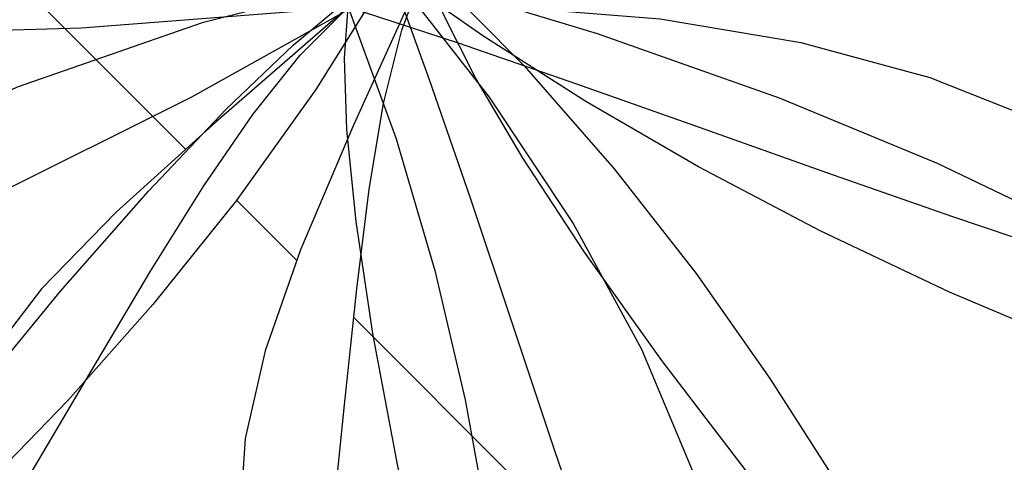
# Model space of a CAD drawing. Units: inches. Extents: x 3590 to 5167, y 65 to 1917.
# Tile 74 of 100: x 5045.84 to 5058.39, y 1773.22 to 1778.86. Entities that reach past the tile are written whole.
import ezdxf

# ---------------------------------------------------------------- set-up
doc = ezdxf.new("R2010")
doc.units = ezdxf.units.IN
for name, color, linetype, lineweight in [('A-ANNO-DIMS', 2, 'Continuous', 18), ('A-FLOR-PATT', 8, 'Continuous', 13), ('L-PLNT', 94, 'Continuous', 18)]:
    doc.layers.add(name, color=color, linetype=linetype, lineweight=lineweight)
doc.layers.add('DIENHOA', color=3, linetype='Continuous')
doc.styles.get("Standard").update_dxf_attribs({"font": 'arial.ttf'})
doc.dimstyles.new('ISO-25', dxfattribs={"dimtxt": 9, "dimasz": 2.5, "dimexe": 1.25, "dimexo": 0.625, "dimtad": 1, "dimdec": 1, "dimlunit": 3, "dimtxsty": 'Standard', "dimcen": 2.5, "dimadec": 0, "dimazin": 0, "dimtfac": 1, "dimtdec": 1, "dimtmove": 0, "dimatfit": 3, "dimfxl": 1, "dimarcsym": 0})

# ---------------------------------------------------------------- blocks, each defined once
blk = doc.blocks.new('Cay03_mb')
at = {"layer": 'DIENHOA'}
for p, q in [((5.39, -7.78), (-33.18, -69.47)), ((5.39, -7.78), (56.83, -73.35)), ((25.88, -64.38), (5.39, -7.78)), ((5.39, -7.78), (112.81, -40.3)), ((53.47, -41.58), (5.39, -7.78)), ((-45.06, -46.34), (-16.51, -22.43)), ((112.81, -40.3), (207.46, -73.81)), ((106.98, -75.69), (53.47, -41.58)), ((-79.78, -79.55), (-45.06, -46.34)), ((47.05, -125.9), (25.88, -64.38)), ((-33.18, -69.47), (-74.57, -127.29)), ((56.83, -73.35), (100.42, -139.07)), ((165.52, -109.6), (106.98, -75.69)), ((207.46, -73.81), (289.55, -107.64)), ((-120.2, -122.13), (-79.78, -79.55)), ((228.67, -142.77), (165.52, -109.6)), ((289.55, -107.64), (359.29, -141.1)), ((-165.86, -174.12), (-120.2, -122.13)), ((-74.57, -127.29), (-117.85, -181.14)), ((68.74, -190.55), (47.05, -125.9)), ((100.42, -139.07), (135.85, -204.28)), ((296, -174.69), (228.67, -142.77)), ((-216.28, -235.58), (-165.86, -174.12)), ((367.1, -204.83), (296, -174.69)), ((-117.85, -181.14), (-162.07, -230.91)), ((90.79, -256.57), (68.74, -190.55)), ((135.85, -204.28), (162.8, -268.28)), ((-162.07, -230.91), (-206.29, -276.49)), ((113.06, -322.16), (90.79, -256.57))]:
    blk.add_line(p, q, dxfattribs=at)
for points in [[(-471.89, -320.34), (-310.46, -179.32), (-97.66, -73.3), (23.69, -5.44)], [(23.69, -5.44), (-92.3, -34.76), (-188.42, -68.2), (-266.88, -105.14), (-329.9, -144.95), (-379.7, -187), (-418.48, -230.67), (-448.47, -275.32), (-471.89, -320.34)], [(23.69, -5.44), (-13.63, -87.94), (-41.14, -152.63), (-59.64, -205.04), (-69.94, -250.66), (-72.84, -295), (-69.17, -343.58), (-59.73, -401.89), (-45.32, -475.45)], [(-45.32, -475.45), (-34.09, -383.24), (-25.4, -302.82), (-18.34, -233.08), (-12.02, -172.9), (-5.55, -121.16), (1.96, -76.75), (11.41, -38.55), (23.69, -5.44)], [(316.49, -418.14), (251.44, -342.76), (194.84, -273.28), (146.52, -210.16), (106.33, -153.83), (74.11, -104.75), (49.71, -63.36), (32.95, -30.11), (23.69, -5.44)], [(23.69, -5.44), (74.94, -57.08), (121.78, -110.58), (164.32, -165.02), (202.67, -219.43), (236.95, -272.89), (267.27, -324.46), (293.75, -373.19), (316.49, -418.14)], [(-598.36, -104.66), (-392.67, -44.38), (-155.01, -37.42), (-16.39, -26.73)], [(-276.22, -424.43), (-227.35, -345.43), (-185.71, -276.08), (-150.05, -215.74), (-119.06, -163.76), (-91.49, -119.51), (-66.04, -82.35), (-41.43, -51.64), (-16.39, -26.73)], [(-16.39, -26.73), (-84.88, -85.96), (-136.99, -133.15), (-175.77, -172.96), (-204.26, -210.05), (-225.5, -249.08), (-242.55, -294.71), (-258.44, -351.61), (-276.22, -424.43)], [(76.25, -524.2), (48.83, -428.48), (26.6, -341.67), (9.22, -264.1), (-3.63, -196.11), (-12.28, -138.04), (-17.07, -90.23), (-18.33, -53.01), (-16.39, -26.73)], [(-16.39, -26.73), (66.95, -26.58), (145.58, -32.71), (218.77, -44.94), (285.79, -63.12), (345.92, -87.06), (398.42, -116.6), (442.57, -151.57), (477.63, -191.79)], [(477.63, -191.79), (421.82, -176.03), (361.32, -156.94), (297.62, -135.49), (232.22, -112.64), (166.63, -89.37), (102.33, -66.65), (40.82, -45.45), (-16.39, -26.73)], [(-16.39, -26.73), (8.47, -95.11), (28.54, -163.33), (44.32, -230.59), (56.3, -296.08), (64.99, -358.99), (70.88, -418.52), (74.46, -473.86), (76.25, -524.2)]]:
    blk.add_lwpolyline(points, dxfattribs=at)
blk = doc.blocks.new('*D322')
at = {"layer": 'A-ANNO-DIMS', "color": 0, "lineweight": -2, "transparency": 16777216}
for p, q in [((5035.744, 1766.184), (5035.744, 1761.199)), ((5064.812, 1766.184), (5064.812, 1761.199)), ((5038.244, 1762.449), (5062.312, 1762.449)), ((5064.812, 1762.449), (5166.991, 1762.449))]:
    blk.add_line(p, q, dxfattribs=at)
at = {"layer": 'A-ANNO-DIMS', "color": 0, "transparency": 16777216}
for points in [[(5038.244, 1762.866), (5038.244, 1762.032), (5035.744, 1762.449)], [(5062.312, 1762.866), (5062.312, 1762.032), (5064.812, 1762.449)]]:
    blk.add_solid(points, dxfattribs=at)
at = {"layer": 'Defpoints', "color": 0, "transparency": 16777216}
for p in [(5035.744, 1766.809), (5064.812, 1766.809), (5064.812, 1762.449)]:
    blk.add_point(p, dxfattribs=at)
at = {"layer": 'A-ANNO-DIMS', "color": 0, "transparency": 16777216, "insert": (5117.152, 1767.669), "char_height": 9, "attachment_point": 5}
blk.add_mtext('PLANT 2\'-5" TYP.', dxfattribs=at)
blk = doc.blocks.new('*D323')
at = {"layer": 'A-ANNO-DIMS', "color": 0, "lineweight": -2, "transparency": 16777216}
for p, q in [((5069.172, 1795.216), (5069.172, 1874.95)), ((5065.437, 1795.216), (5070.422, 1795.216)), ((5069.172, 1769.309), (5069.172, 1792.716)), ((5065.437, 1766.809), (5070.422, 1766.809))]:
    blk.add_line(p, q, dxfattribs=at)
at = {"layer": 'A-ANNO-DIMS', "color": 0, "transparency": 16777216}
for points in [[(5068.756, 1792.716), (5069.589, 1792.716), (5069.172, 1795.216)], [(5068.756, 1769.309), (5069.589, 1769.309), (5069.172, 1766.809)]]:
    blk.add_solid(points, dxfattribs=at)
at = {"layer": 'Defpoints', "color": 0, "transparency": 16777216}
for p in [(5064.812, 1795.216), (5069.172, 1795.216), (5064.812, 1766.809)]:
    blk.add_point(p, dxfattribs=at)
at = {"layer": 'A-ANNO-DIMS', "color": 0, "transparency": 16777216, "insert": (5063.894, 1836.333), "char_height": 9, "attachment_point": 5, "rotation": 90}
blk.add_mtext('2\'-4 1/2" TYP.', dxfattribs=at)

msp = doc.modelspace()

# ---------------------------------------------------------------- hatches: boundary and pattern name
at = {"layer": 'A-FLOR-PATT', "transparency": 33554687}
h = msp.add_hatch(dxfattribs=at)
h.set_pattern_fill('AR-HBONE', color=256, scale=0.2)
h.set_pattern_definition([(45, (-588.972, 0), (0, 28.73682), [60.96, -20.32]), (135, (-574.604, 14.368), (3e-15, 28.73682), [60.96, -20.32])])
h.paths.add_polyline_path([(5071.274, 1796.999), (4933.274, 1796.999), (4933.274, 1753.999), (4962.774, 1753.999, -0.414214), (4928.774, 1719.999), (4933.274, 1718.999), (4933.274, 1334.999), (5071.274, 1334.999)])
h.paths.add_polyline_path([(4951.78, 1521.077), (4951.715, 1521.04), (4951.563, 1520.895)], flags=16)
h.paths.add_polyline_path([(4952.267, 1521.376), (4952.198, 1521.371), (4952.198, 1521.356)], flags=0)
h.paths.add_polyline_path([(4967.051, 1529.728), (4965.231, 1528.694), (4963.411, 1527.714), (4961.756, 1526.851), (4963.589, 1527.449), (4964.036, 1527.478), (4962.975, 1527.249), (4961.76, 1526.852), (4959.792, 1525.834), (4958.005, 1524.895), (4956.24, 1523.93), (4954.504, 1522.919), (4954.129, 1522.682), (4953.361, 1521.997), (4953.366, 1521.998), (4953.605, 1522.064), (4955.106, 1522.761), (4956.921, 1523.434), (4958.678, 1523.915), (4960.358, 1524.2), (4961.945, 1524.286), (4964.171, 1524.108), (4965.958, 1523.309), (4963.863, 1522.976), (4965.187, 1522.499), (4963.366, 1522.497), (4961.545, 1522.487), (4959.764, 1522.461), (4958.304, 1522.419), (4957.974, 1522.388), (4956.307, 1522.232), (4954.718, 1522.071), (4953.251, 1521.899), (4953.525, 1521.623), (4954.331, 1521.379), (4956.243, 1521.23), (4958.039, 1520.93), (4959.684, 1520.483), (4961.16, 1519.896), (4963.107, 1518.8), (4964.393, 1517.325), (4962.973, 1517.726), (4964.558, 1516.661), (4965.407, 1515.708), (4963.507, 1516.322), (4961.68, 1517.005), (4959.935, 1517.745), (4958.282, 1518.528), (4956.732, 1519.343), (4955.295, 1520.175), (4954.672, 1520.572), (4954.513, 1520.627), (4955.658, 1519.318), (4956.703, 1517.982), (4957.644, 1516.647), (4958.485, 1515.334), (4959.55, 1513.524), (4960.438, 1511.769), (4958.841, 1513.62), (4957.452, 1515.325), (4955.819, 1517.459), (4956.665, 1515.448), (4957.111, 1513.923), (4957.447, 1511.714), (4957.076, 1509.793), (4956.538, 1511.11), (4955.992, 1512.569), (4955.444, 1514.125), (4954.898, 1515.735), (4954.357, 1517.356), (4953.824, 1518.943), (4953.305, 1520.452), (4953.065, 1521.116), (4952.971, 1521.146), (4952.949, 1521.086), (4952.73, 1520.199), (4953.37, 1518.024), (4953.757, 1516.373), (4954.051, 1514.765), (4954.264, 1513.221), (4954.471, 1511.131), (4954.497, 1510.402), (4954.409, 1511.76), (4954.264, 1513.221), (4954.051, 1514.765), (4953.757, 1516.373), (4953.37, 1518.024), (4952.877, 1519.698), (4952.716, 1520.141), (4952.533, 1519.059), (4952.374, 1517.789), (4952.219, 1516.312), (4952.046, 1514.6), (4951.833, 1512.626), (4951.557, 1510.363), (4951.203, 1512.168), (4950.852, 1514.339), (4950.985, 1516.376), (4951.66, 1518.286), (4952.593, 1520.481), (4952.357, 1521.13), (4951.855, 1520.328), (4950.839, 1518.908), (4949.777, 1517.587), (4948.916, 1516.617), (4948.111, 1515.256), (4947.089, 1513.554), (4945.889, 1511.615), (4946.326, 1513.402), (4946.562, 1514.249), (4945.528, 1513.327), (4944.581, 1512.531), (4946.018, 1514.508), (4947.204, 1516.048), (4947.893, 1517.313), (4949.307, 1518.764), (4950.414, 1519.767), (4950.451, 1519.806), (4952.267, 1521.376), (4951.645, 1521.493), (4950.404, 1521.18), (4948.044, 1520.359), (4946.119, 1519.452), (4944.572, 1518.475), (4943.35, 1517.443), (4941.997, 1515.92), (4941.661, 1515.275), (4942.813, 1516.99), (4944.572, 1518.475), (4946.119, 1519.452), (4948.044, 1520.359), (4950.404, 1521.18), (4951.645, 1521.493), (4949.647, 1521.868), (4948.6, 1521.756), (4947.126, 1521.57), (4945.42, 1521.348), (4943.45, 1521.105), (4941.183, 1520.856), (4942.86, 1521.613), (4943.873, 1522.03), (4942.952, 1521.909), (4941.41, 1521.485), (4939.543, 1520.67), (4938.968, 1520.226), (4940.733, 1521.299), (4942.952, 1521.909), (4943.702, 1522.008), (4945.894, 1522.7), (4947.565, 1522.714), (4948.921, 1522.566), (4951.131, 1522.183), (4950.971, 1522.297), (4948.129, 1523.006), (4946.035, 1523.707), (4944.232, 1524.521), (4942.707, 1525.461), (4941.444, 1526.537), (4940.43, 1527.761), (4939.649, 1529.143), (4941.421, 1528.122), (4943.147, 1527.132), (4944.841, 1526.175), (4946.514, 1525.25), (4948.179, 1524.359), (4948.365, 1524.263), (4946.475, 1526.045), (4945.181, 1527.54), (4944.19, 1529.033), (4943.496, 1530.54), (4943.278, 1531.36), (4942.498, 1531.919), (4943.114, 1531.762), (4942.959, 1533.659), (4944.14, 1531.989), (4944.612, 1531.323), (4946.202, 1530.463), (4947.486, 1529.509), (4948.79, 1528.226), (4950.368, 1526.237), (4949.485, 1528.155), (4948.851, 1530.123), (4948.491, 1532.041), (4948.381, 1533.918), (4948.501, 1535.76), (4948.827, 1537.573), (4949.418, 1535.565), (4949.957, 1533.569), (4950.464, 1531.586), (4950.961, 1529.617), (4951.391, 1527.954), (4951.724, 1530.687), (4952.201, 1532.58), (4952.889, 1534.33), (4953.77, 1535.951), (4954.827, 1537.46), (4954.521, 1535.39), (4954.273, 1533.937), (4955.58, 1535.663), (4956.748, 1536.739), (4956.159, 1534.78), (4955.589, 1532.873), (4955.043, 1531.006), (4954.525, 1529.166), (4954.038, 1527.341), (4953.638, 1525.733), (4953.611, 1525.586), (4953.398, 1524.166), (4953.382, 1524.009), (4954.07, 1525.476), (4954.912, 1527.022), (4956.136, 1528.894), (4957.847, 1530.577), (4959.376, 1531.54), (4958.256, 1530.104), (4957.143, 1528.663), (4956.066, 1527.243), (4955.056, 1525.871), (4954.141, 1524.571), (4953.352, 1523.372), (4953.311, 1523.303), (4953.273, 1522.925), (4953.261, 1522.382), (4954.103, 1523.373), (4954.63, 1524.284), (4955.961, 1526.358), (4957.23, 1528.13), (4958.421, 1529.609), (4960.037, 1531.368), (4961.374, 1532.375), (4962.101, 1532.77), (4961.07, 1531.061), (4959.987, 1529.438), (4958.869, 1527.908), (4958.15, 1527.007), (4959.803, 1528.003), (4961.589, 1528.793), (4963.391, 1529.328), (4965.211, 1529.632)], flags=16)
h.paths.add_polyline_path([(4962.944, 1523.182), (4961.107, 1523.422), (4960.392, 1523.362), (4962.35, 1523.331)], flags=0)
h.paths.add_polyline_path([(5049.541, 1584.551), (5049.476, 1584.515), (5049.325, 1584.37)], flags=16)
h.paths.add_polyline_path([(5050.028, 1584.851), (5049.959, 1584.845), (5049.959, 1584.83)], flags=0)
h.paths.add_polyline_path([(5042.333, 1581.949), (5043.88, 1582.926), (5045.806, 1583.833), (5048.165, 1584.654), (5049.406, 1584.967), (5047.408, 1585.342), (5046.361, 1585.231), (5044.888, 1585.044), (5043.181, 1584.822), (5041.211, 1584.579), (5038.944, 1584.33), (5040.622, 1585.087), (5041.634, 1585.504), (5040.713, 1585.383), (5039.171, 1584.959), (5037.304, 1584.144), (5036.729, 1583.7), (5038.494, 1584.773), (5040.713, 1585.383), (5041.463, 1585.482), (5043.655, 1586.174), (5045.326, 1586.188), (5046.682, 1586.04), (5048.893, 1585.657), (5048.732, 1585.771), (5045.891, 1586.48), (5043.796, 1587.181), (5041.994, 1587.996), (5040.468, 1588.935), (5039.205, 1590.011), (5038.191, 1591.235), (5037.41, 1592.617), (5039.182, 1591.596), (5040.909, 1590.607), (5042.602, 1589.649), (5044.275, 1588.724), (5045.94, 1587.833), (5046.126, 1587.738), (5044.237, 1589.519), (5042.942, 1591.015), (5041.952, 1592.508), (5041.257, 1594.014), (5041.039, 1594.834), (5040.26, 1595.393), (5040.875, 1595.237), (5040.721, 1597.133), (5041.901, 1595.463), (5042.373, 1594.798), (5043.963, 1593.938), (5045.247, 1592.983), (5046.552, 1591.701), (5048.129, 1589.712), (5047.247, 1591.63), (5046.613, 1593.597), (5046.252, 1595.515), (5046.142, 1597.392), (5046.262, 1599.234), (5046.588, 1601.047), (5047.179, 1599.039), (5047.718, 1597.043), (5048.225, 1595.06), (5048.722, 1593.091), (5049.152, 1591.429), (5049.485, 1594.161), (5049.962, 1596.054), (5050.65, 1597.804), (5051.532, 1599.425), (5052.589, 1600.934), (5052.283, 1598.864), (5052.034, 1597.411), (5053.341, 1599.137), (5054.509, 1600.213), (5053.92, 1598.254), (5053.35, 1596.348), (5052.805, 1594.48), (5052.286, 1592.64), (5051.799, 1590.815), (5051.4, 1589.207), (5051.373, 1589.06), (5051.159, 1587.64), (5051.143, 1587.483), (5051.831, 1588.95), (5052.673, 1590.496), (5053.898, 1592.368), (5055.608, 1594.051), (5057.137, 1595.014), (5056.017, 1593.578), (5054.904, 1592.137), (5053.828, 1590.717), (5052.817, 1589.345), (5051.902, 1588.046), (5051.113, 1586.846), (5051.072, 1586.777), (5051.034, 1586.399), (5051.022, 1585.856), (5051.864, 1586.847), (5052.391, 1587.758), (5053.723, 1589.832), (5054.991, 1591.604), (5056.182, 1593.083), (5057.798, 1594.842), (5059.135, 1595.849), (5059.863, 1596.244), (5058.831, 1594.535), (5057.749, 1592.912), (5056.63, 1591.382), (5055.912, 1590.482), (5057.564, 1591.477), (5059.35, 1592.267), (5061.152, 1592.802), (5062.972, 1593.106), (5064.812, 1593.203), (5062.992, 1592.169), (5061.172, 1591.188), (5059.518, 1590.325), (5061.35, 1590.924), (5061.797, 1590.952), (5060.737, 1590.723), (5059.521, 1590.326), (5057.553, 1589.308), (5055.766, 1588.369), (5054.002, 1587.404), (5052.265, 1586.393), (5051.891, 1586.156), (5051.122, 1585.471), (5051.127, 1585.472), (5051.366, 1585.538), (5052.867, 1586.235), (5054.682, 1586.908), (5056.439, 1587.389), (5058.12, 1587.675), (5059.706, 1587.76), (5061.933, 1587.583), (5063.719, 1586.783), (5061.624, 1586.45), (5062.949, 1585.973), (5061.127, 1585.971), (5059.307, 1585.961), (5057.525, 1585.935), (5056.065, 1585.893), (5055.735, 1585.862), (5054.068, 1585.707), (5052.479, 1585.546), (5051.012, 1585.373), (5051.286, 1585.097), (5052.092, 1584.853), (5054.004, 1584.704), (5055.8, 1584.404), (5057.446, 1583.958), (5058.921, 1583.37), (5060.868, 1582.274), (5062.154, 1580.799), (5060.734, 1581.2), (5062.32, 1580.135), (5063.168, 1579.182), (5061.269, 1579.796), (5059.441, 1580.479), (5057.696, 1581.219), (5056.043, 1582.003), (5054.493, 1582.817), (5053.057, 1583.649), (5052.433, 1584.047), (5052.274, 1584.101), (5053.42, 1582.793), (5054.464, 1581.457), (5055.405, 1580.121), (5056.247, 1578.809), (5057.311, 1576.998), (5058.199, 1575.244), (5056.602, 1577.094), (5055.213, 1578.799), (5053.58, 1580.933), (5054.427, 1578.922), (5054.872, 1577.397), (5055.208, 1575.189), (5054.838, 1573.267), (5054.299, 1574.584), (5053.754, 1576.043), (5053.206, 1577.599), (5052.659, 1579.209), (5052.118, 1580.83), (5051.585, 1582.417), (5051.066, 1583.927), (5050.826, 1584.59), (5050.733, 1584.62), (5050.711, 1584.561), (5050.491, 1583.673), (5051.131, 1581.498), (5051.518, 1579.847), (5051.813, 1578.24), (5052.026, 1576.695), (5052.233, 1574.605), (5052.258, 1573.876), (5052.17, 1575.234), (5052.026, 1576.695), (5051.813, 1578.24), (5051.518, 1579.847), (5051.131, 1581.498), (5050.638, 1583.172), (5050.477, 1583.615), (5050.294, 1582.533), (5050.136, 1581.263), (5049.981, 1579.786), (5049.807, 1578.074), (5049.594, 1576.1), (5049.318, 1573.837), (5048.965, 1575.642), (5048.613, 1577.813), (5048.747, 1579.85), (5049.421, 1581.76), (5050.354, 1583.955), (5050.118, 1584.604), (5049.616, 1583.802), (5048.6, 1582.382), (5047.538, 1581.061), (5046.677, 1580.091), (5045.872, 1578.73), (5044.85, 1577.028), (5043.651, 1575.089), (5044.087, 1576.877), (5044.324, 1577.723), (5043.289, 1576.801), (5042.342, 1576.005), (5043.779, 1577.982), (5044.966, 1579.522), (5045.655, 1580.787), (5047.068, 1582.239), (5048.175, 1583.241), (5048.213, 1583.28), (5050.028, 1584.851), (5049.406, 1584.967), (5048.165, 1584.654), (5045.806, 1583.833), (5043.88, 1582.926), (5042.333, 1581.949), (5041.111, 1580.917), (5039.758, 1579.394), (5039.423, 1578.749), (5040.575, 1580.464)], flags=16)
h.paths.add_polyline_path([(4954.799, 1533.12), (4954.262, 1532.079), (4953.831, 1530.935), (4953.505, 1529.636), (4953.283, 1528.133), (4953.167, 1526.376), (4953.156, 1524.315), (4953.277, 1521.236), (4952.802, 1521.842), (4951.557, 1521.998), (4950.976, 1521.961), (4952.661, 1521.941), (4952.802, 1521.842), (4953.152, 1523.593), (4953.167, 1526.376), (4953.283, 1528.133), (4953.609, 1530.346), (4954.456, 1532.592)], flags=0)
h.paths.add_polyline_path([(5050.563, 1585.316), (5049.318, 1585.472), (5048.737, 1585.435), (5050.422, 1585.415), (5050.563, 1585.316), (5050.914, 1587.067), (5050.928, 1589.851), (5051.045, 1591.607), (5051.371, 1593.82), (5052.217, 1596.066), (5052.56, 1596.594), (5052.024, 1595.554), (5051.592, 1594.409), (5051.266, 1593.11), (5051.045, 1591.607), (5050.928, 1589.851), (5050.918, 1587.789), (5051.038, 1584.71)], flags=0)
h.paths.add_polyline_path([(5058.153, 1586.836), (5060.111, 1586.805), (5060.705, 1586.656), (5058.868, 1586.896)], flags=0)
h.paths.add_polyline_path([(5049.541, 1430.936), (5049.476, 1430.9), (5049.325, 1430.755)], flags=16)
h.paths.add_polyline_path([(5050.028, 1431.236), (5049.959, 1431.231), (5049.959, 1431.215)], flags=0)
h.paths.add_polyline_path([(5046.588, 1447.432), (5047.179, 1445.425), (5047.718, 1443.429), (5048.225, 1441.446), (5048.722, 1439.476), (5049.152, 1437.814), (5049.485, 1440.546), (5049.962, 1442.439), (5050.65, 1444.189), (5051.532, 1445.811), (5052.589, 1447.319), (5052.283, 1445.249), (5052.034, 1443.796), (5053.341, 1445.522), (5054.509, 1446.598), (5053.92, 1444.64), (5053.35, 1442.733), (5052.805, 1440.865), (5052.286, 1439.025), (5051.799, 1437.201), (5051.4, 1435.592), (5051.373, 1435.445), (5051.159, 1434.025), (5051.143, 1433.868), (5051.831, 1435.335), (5052.673, 1436.881), (5053.898, 1438.753), (5055.608, 1440.436), (5057.137, 1441.4), (5056.017, 1439.963), (5054.904, 1438.522), (5053.828, 1437.102), (5052.817, 1435.73), (5051.902, 1434.431), (5051.113, 1433.231), (5051.072, 1433.162), (5051.034, 1432.784), (5051.022, 1432.242), (5051.864, 1433.232), (5052.391, 1434.143), (5053.723, 1436.217), (5054.991, 1437.989), (5056.182, 1439.468), (5057.798, 1441.227), (5059.135, 1442.235), (5059.863, 1442.629), (5058.831, 1440.921), (5057.749, 1439.298), (5056.63, 1437.767), (5055.912, 1436.867), (5057.564, 1437.863), (5059.35, 1438.652), (5061.152, 1439.187), (5062.972, 1439.491), (5064.812, 1439.588), (5062.992, 1438.554), (5061.172, 1437.573), (5059.518, 1436.71), (5061.35, 1437.309), (5061.797, 1437.337), (5060.737, 1437.108), (5059.521, 1436.711), (5057.553, 1435.693), (5055.766, 1434.754), (5054.002, 1433.789), (5052.265, 1432.778), (5051.891, 1432.541), (5051.122, 1431.856), (5051.127, 1431.857), (5051.366, 1431.923), (5052.867, 1432.62), (5054.682, 1433.293), (5056.439, 1433.775), (5058.12, 1434.06), (5059.706, 1434.145), (5061.933, 1433.968), (5063.719, 1433.168), (5061.624, 1432.835), (5062.949, 1432.358), (5061.127, 1432.357), (5059.307, 1432.346), (5057.525, 1432.32), (5056.065, 1432.278), (5055.735, 1432.248), (5054.068, 1432.092), (5052.479, 1431.931), (5051.012, 1431.759), (5051.286, 1431.482), (5052.092, 1431.238), (5054.004, 1431.089), (5055.8, 1430.789), (5057.446, 1430.343), (5058.921, 1429.755), (5060.868, 1428.66), (5062.154, 1427.185), (5060.734, 1427.585), (5062.32, 1426.52), (5063.168, 1425.567), (5061.269, 1426.181), (5059.441, 1426.865), (5057.696, 1427.604), (5056.043, 1428.388), (5054.493, 1429.202), (5053.057, 1430.034), (5052.433, 1430.432), (5052.274, 1430.487), (5053.42, 1429.178), (5054.464, 1427.842), (5055.405, 1426.506), (5056.247, 1425.194), (5057.311, 1423.383), (5058.199, 1421.629), (5056.602, 1423.479), (5055.213, 1425.184), (5053.58, 1427.318), (5054.427, 1425.307), (5054.872, 1423.782), (5055.208, 1421.574), (5054.838, 1419.652), (5054.299, 1420.97), (5053.754, 1422.428), (5053.206, 1423.984), (5052.659, 1425.595), (5052.118, 1427.215), (5051.585, 1428.802), (5051.066, 1430.312), (5050.826, 1430.975), (5050.733, 1431.005), (5050.711, 1430.946), (5050.491, 1430.058), (5051.131, 1427.883), (5051.518, 1426.232), (5051.813, 1424.625), (5052.026, 1423.081), (5052.233, 1420.991), (5052.258, 1420.261), (5052.17, 1421.619), (5052.026, 1423.081), (5051.813, 1424.625), (5051.518, 1426.232), (5051.131, 1427.883), (5050.638, 1429.558), (5050.477, 1430.001), (5050.294, 1428.918), (5050.136, 1427.648), (5049.981, 1426.171), (5049.807, 1424.459), (5049.594, 1422.485), (5049.318, 1420.222), (5048.965, 1422.028), (5048.613, 1424.199), (5048.747, 1426.235), (5049.421, 1428.146), (5050.354, 1430.34), (5050.118, 1430.989), (5049.616, 1430.187), (5048.6, 1428.768), (5047.538, 1427.446), (5046.677, 1426.477), (5045.872, 1425.116), (5044.85, 1423.413), (5043.651, 1421.474), (5044.087, 1423.262), (5044.324, 1424.109), (5043.289, 1423.186), (5042.342, 1422.391), (5043.779, 1424.368), (5044.966, 1425.907), (5045.655, 1427.173), (5047.068, 1428.624), (5048.175, 1429.627), (5048.213, 1429.666), (5050.028, 1431.236), (5049.406, 1431.353), (5048.165, 1431.039), (5045.806, 1430.218), (5043.88, 1429.311), (5042.333, 1428.334), (5041.111, 1427.302), (5039.758, 1425.779), (5039.423, 1425.134), (5040.575, 1426.849), (5042.333, 1428.334), (5043.88, 1429.311), (5045.806, 1430.218), (5048.165, 1431.039), (5049.406, 1431.353), (5047.408, 1431.727), (5046.361, 1431.616), (5044.888, 1431.429), (5043.181, 1431.207), (5041.211, 1430.964), (5038.944, 1430.715), (5040.622, 1431.472), (5041.634, 1431.89), (5040.713, 1431.769), (5039.171, 1431.345), (5037.304, 1430.53), (5036.729, 1430.085), (5038.494, 1431.158), (5040.713, 1431.769), (5041.463, 1431.867), (5043.655, 1432.559), (5045.326, 1432.573), (5046.682, 1432.425), (5048.893, 1432.042), (5048.732, 1432.156), (5045.891, 1432.865), (5043.796, 1433.566), (5041.994, 1434.381), (5040.468, 1435.321), (5039.205, 1436.396), (5038.191, 1437.62), (5037.41, 1439.002), (5039.182, 1437.982), (5040.909, 1436.992), (5042.602, 1436.034), (5044.275, 1435.109), (5045.94, 1434.218), (5046.126, 1434.123), (5044.237, 1435.904), (5042.942, 1437.4), (5041.952, 1438.893), (5041.257, 1440.399), (5041.039, 1441.219), (5040.26, 1441.778), (5040.875, 1441.622), (5040.721, 1443.518), (5041.901, 1441.848), (5042.373, 1441.183), (5043.963, 1440.323), (5045.247, 1439.369), (5046.552, 1438.086), (5048.129, 1436.097), (5047.247, 1438.015), (5046.613, 1439.982), (5046.252, 1441.901), (5046.142, 1443.778), (5046.262, 1445.619)], flags=16)
h.paths.add_polyline_path([(5052.382, 1444.255), (5051.623, 1442.78), (5052.024, 1441.939), (5052.56, 1442.98)], flags=0)
h.paths.add_polyline_path([(5050.563, 1431.701), (5049.318, 1431.857), (5048.737, 1431.821), (5050.422, 1431.8)], flags=0)
h.paths.add_polyline_path([(5058.153, 1433.221), (5060.111, 1433.19), (5060.705, 1433.041), (5058.868, 1433.281)], flags=0)
h.paths.add_polyline_path([(5049.541, 1352.285), (5049.476, 1352.249), (5049.325, 1352.104)], flags=16)
h.paths.add_polyline_path([(5050.028, 1352.585), (5049.959, 1352.58), (5049.959, 1352.564)], flags=0)
h.paths.add_polyline_path([(5046.588, 1368.781), (5047.179, 1366.774), (5047.718, 1364.778), (5048.225, 1362.795), (5048.722, 1360.825), (5049.152, 1359.163), (5049.485, 1361.896), (5049.962, 1363.789), (5050.65, 1365.538), (5051.532, 1367.16), (5052.589, 1368.669), (5052.283, 1366.598), (5052.034, 1365.145), (5053.341, 1366.871), (5054.509, 1367.947), (5053.92, 1365.989), (5053.35, 1364.082), (5052.805, 1362.214), (5052.286, 1360.374), (5051.799, 1358.55), (5051.4, 1356.942), (5051.373, 1356.794), (5051.159, 1355.374), (5051.143, 1355.218), (5051.831, 1356.684), (5052.673, 1358.23), (5053.898, 1360.102), (5055.608, 1361.786), (5057.137, 1362.749), (5056.017, 1361.313), (5054.904, 1359.872), (5053.828, 1358.452), (5052.817, 1357.079), (5051.902, 1355.78), (5051.113, 1354.581), (5051.072, 1354.512), (5051.034, 1354.133), (5051.022, 1353.591), (5051.864, 1354.581), (5052.391, 1355.492), (5053.723, 1357.566), (5054.991, 1359.338), (5056.182, 1360.817), (5057.798, 1362.577), (5059.135, 1363.584), (5059.863, 1363.979), (5058.831, 1362.27), (5057.749, 1360.647), (5056.63, 1359.117), (5055.912, 1358.216), (5057.564, 1359.212), (5059.35, 1360.001), (5061.152, 1360.536), (5062.972, 1360.841), (5064.812, 1360.937), (5062.992, 1359.903), (5061.172, 1358.923), (5059.518, 1358.059), (5061.35, 1358.658), (5061.797, 1358.687), (5060.737, 1358.458), (5059.521, 1358.061), (5057.553, 1357.043), (5055.766, 1356.103), (5054.002, 1355.138), (5052.265, 1354.127), (5051.891, 1353.89), (5051.122, 1353.206), (5051.127, 1353.206), (5051.366, 1353.272), (5052.867, 1353.969), (5054.682, 1354.643), (5056.439, 1355.124), (5058.12, 1355.409), (5059.706, 1355.495), (5061.933, 1355.317), (5063.719, 1354.518), (5061.624, 1354.184), (5062.949, 1353.708), (5061.127, 1353.706), (5059.307, 1353.695), (5057.525, 1353.669), (5056.065, 1353.627), (5055.735, 1353.597), (5054.068, 1353.441), (5052.479, 1353.28), (5051.012, 1353.108), (5051.286, 1352.831), (5052.092, 1352.587), (5054.004, 1352.439), (5055.8, 1352.138), (5057.446, 1351.692), (5058.921, 1351.104), (5060.868, 1350.009), (5062.154, 1348.534), (5060.734, 1348.935), (5062.32, 1347.869), (5063.168, 1346.916), (5061.269, 1347.53), (5059.441, 1348.214), (5057.696, 1348.954), (5056.043, 1349.737), (5054.493, 1350.551), (5053.057, 1351.383), (5052.433, 1351.781), (5052.274, 1351.836), (5053.42, 1350.527), (5054.464, 1349.191), (5055.405, 1347.855), (5056.247, 1346.543), (5057.311, 1344.733), (5058.199, 1342.978), (5056.602, 1344.828), (5055.213, 1346.534), (5053.58, 1348.667), (5054.427, 1346.656), (5054.872, 1345.132), (5055.208, 1342.923), (5054.838, 1341.002), (5054.299, 1342.319), (5053.754, 1343.778), (5053.206, 1345.334), (5052.659, 1346.944), (5052.118, 1348.564), (5051.585, 1350.151), (5051.066, 1351.661), (5050.826, 1352.324), (5050.733, 1352.355), (5050.711, 1352.295), (5050.491, 1351.408), (5051.131, 1349.232), (5051.518, 1347.581), (5051.813, 1345.974), (5052.026, 1344.43), (5052.233, 1342.34), (5052.258, 1341.61), (5052.17, 1342.969), (5052.026, 1344.43), (5051.813, 1345.974), (5051.518, 1347.581), (5051.131, 1349.232), (5050.638, 1350.907), (5050.477, 1351.35), (5050.294, 1350.267), (5050.136, 1348.997), (5049.981, 1347.52), (5049.807, 1345.809), (5049.594, 1343.835), (5049.318, 1341.571), (5048.965, 1343.377), (5048.613, 1345.548), (5048.747, 1347.585), (5049.421, 1349.495), (5050.354, 1351.689), (5050.118, 1352.339), (5049.616, 1351.536), (5048.6, 1350.117), (5047.538, 1348.795), (5046.677, 1347.826), (5045.872, 1346.465), (5044.85, 1344.763), (5043.651, 1342.824), (5044.087, 1344.611), (5044.324, 1345.458), (5043.289, 1344.535), (5042.342, 1343.74), (5043.779, 1345.717), (5044.966, 1347.256), (5045.655, 1348.522), (5047.068, 1349.973), (5048.175, 1350.976), (5048.213, 1351.015), (5050.028, 1352.585), (5049.406, 1352.702), (5048.165, 1352.388), (5045.806, 1351.567), (5043.88, 1350.661), (5042.333, 1349.683), (5041.111, 1348.651), (5039.758, 1347.128), (5039.423, 1346.483), (5040.575, 1348.198), (5042.333, 1349.683), (5043.88, 1350.661), (5045.806, 1351.567), (5048.165, 1352.388), (5049.406, 1352.702), (5047.408, 1353.076), (5046.361, 1352.965), (5044.888, 1352.779), (5043.181, 1352.556), (5041.211, 1352.313), (5038.944, 1352.065), (5040.622, 1352.821), (5041.634, 1353.239), (5040.713, 1353.118), (5039.171, 1352.694), (5037.304, 1351.879), (5036.729, 1351.434), (5038.494, 1352.508), (5040.713, 1353.118), (5041.463, 1353.216), (5043.655, 1353.909), (5045.326, 1353.923), (5046.682, 1353.774), (5048.893, 1353.391), (5048.732, 1353.506), (5045.891, 1354.214), (5043.796, 1354.915), (5041.994, 1355.73), (5040.468, 1356.67), (5039.205, 1357.746), (5038.191, 1358.969), (5037.41, 1360.352), (5039.182, 1359.331), (5040.909, 1358.341), (5042.602, 1357.383), (5044.275, 1356.458), (5045.94, 1355.567), (5046.126, 1355.472), (5044.237, 1357.253), (5042.942, 1358.749), (5041.952, 1360.242), (5041.257, 1361.748), (5041.039, 1362.568), (5040.26, 1363.128), (5040.875, 1362.971), (5040.721, 1364.867), (5041.901, 1363.197), (5042.373, 1362.532), (5043.963, 1361.672), (5045.247, 1360.718), (5046.552, 1359.435), (5048.129, 1357.446), (5047.247, 1359.364), (5046.613, 1361.331), (5046.252, 1363.25), (5046.142, 1365.127), (5046.262, 1366.969)], flags=16)
h.paths.add_polyline_path([(5052.382, 1365.604), (5051.623, 1364.129), (5052.024, 1363.288), (5052.56, 1364.329)], flags=0)
h.paths.add_polyline_path([(4951.78, 1698.041), (4951.715, 1698.005), (4951.563, 1697.859)], flags=16)
h.paths.add_polyline_path([(4952.267, 1698.341), (4952.198, 1698.335), (4952.198, 1698.32)], flags=0)
h.paths.add_polyline_path([(4957.076, 1686.757), (4956.538, 1688.074), (4955.992, 1689.533), (4955.444, 1691.089), (4954.898, 1692.699), (4954.357, 1694.32), (4953.824, 1695.907), (4953.305, 1697.417), (4953.065, 1698.08), (4952.971, 1698.11), (4952.949, 1698.051), (4952.73, 1697.163), (4953.37, 1694.988), (4953.757, 1693.337), (4954.051, 1691.729), (4954.264, 1690.185), (4954.471, 1688.095), (4954.497, 1687.366), (4954.409, 1688.724), (4954.264, 1690.185), (4954.051, 1691.729), (4953.757, 1693.337), (4953.37, 1694.988), (4952.877, 1696.662), (4952.716, 1697.105), (4952.533, 1696.023), (4952.374, 1694.753), (4952.219, 1693.276), (4952.046, 1691.564), (4951.833, 1689.59), (4951.557, 1687.327), (4951.203, 1689.132), (4950.852, 1691.303), (4950.985, 1693.34), (4951.66, 1695.25), (4952.593, 1697.445), (4952.357, 1698.094), (4951.855, 1697.292), (4950.839, 1695.872), (4949.777, 1694.551), (4948.916, 1693.581), (4948.111, 1692.22), (4947.089, 1690.518), (4945.889, 1688.579), (4946.326, 1690.366), (4946.562, 1691.213), (4945.528, 1690.291), (4944.581, 1689.495), (4946.018, 1691.472), (4947.204, 1693.012), (4947.893, 1694.277), (4949.307, 1695.729), (4950.414, 1696.731), (4950.451, 1696.77), (4952.267, 1698.341), (4951.645, 1698.457), (4950.404, 1698.144), (4948.044, 1697.323), (4946.119, 1696.416), (4944.572, 1695.439), (4943.35, 1694.407), (4941.997, 1692.884), (4941.661, 1692.239), (4942.813, 1693.954), (4944.572, 1695.439), (4946.119, 1696.416), (4948.044, 1697.323), (4950.404, 1698.144), (4951.645, 1698.457), (4949.647, 1698.832), (4948.6, 1698.72), (4947.126, 1698.534), (4945.42, 1698.312), (4943.45, 1698.069), (4941.183, 1697.82), (4942.86, 1698.577), (4943.873, 1698.994), (4942.952, 1698.873), (4941.41, 1698.449), (4939.543, 1697.634), (4938.968, 1697.19), (4940.733, 1698.263), (4942.952, 1698.873), (4943.702, 1698.972), (4945.894, 1699.664), (4947.565, 1699.678), (4948.921, 1699.53), (4951.131, 1699.147), (4950.971, 1699.261), (4948.129, 1699.97), (4946.035, 1700.671), (4944.232, 1701.486), (4942.707, 1702.425), (4941.444, 1703.501), (4940.43, 1704.725), (4939.649, 1706.107), (4941.421, 1705.086), (4943.147, 1704.097), (4944.841, 1703.139), (4946.514, 1702.214), (4948.179, 1701.323), (4948.365, 1701.227), (4946.475, 1703.009), (4945.181, 1704.505), (4944.19, 1705.997), (4943.496, 1707.504), (4943.278, 1708.324), (4942.498, 1708.883), (4943.114, 1708.727), (4942.959, 1710.623), (4944.14, 1708.953), (4944.612, 1708.287), (4946.202, 1707.428), (4947.486, 1706.473), (4948.79, 1705.191), (4950.368, 1703.202), (4949.485, 1705.12), (4948.851, 1707.087), (4948.491, 1709.005), (4948.381, 1710.882), (4948.501, 1712.724), (4948.827, 1714.537), (4949.418, 1712.529), (4949.957, 1710.533), (4950.464, 1708.55), (4950.961, 1706.581), (4951.391, 1704.919), (4951.724, 1707.651), (4952.201, 1709.544), (4952.889, 1711.294), (4953.77, 1712.915), (4954.827, 1714.424), (4954.521, 1712.354), (4954.273, 1710.901), (4955.58, 1712.627), (4956.748, 1713.703), (4956.159, 1711.744), (4955.589, 1709.837), (4955.043, 1707.97), (4954.525, 1706.13), (4954.038, 1704.305), (4953.638, 1702.697), (4953.611, 1702.55), (4953.398, 1701.13), (4953.382, 1700.973), (4954.07, 1702.44), (4954.912, 1703.986), (4956.136, 1705.858), (4957.847, 1707.541), (4959.376, 1708.504), (4958.256, 1707.068), (4957.143, 1705.627), (4956.066, 1704.207), (4955.056, 1702.835), (4954.141, 1701.536), (4953.352, 1700.336), (4953.311, 1700.267), (4953.273, 1699.889), (4953.261, 1699.346), (4954.103, 1700.337), (4954.63, 1701.248), (4955.961, 1703.322), (4957.23, 1705.094), (4958.421, 1706.573), (4960.037, 1708.332), (4961.374, 1709.339), (4962.101, 1709.734), (4961.07, 1708.025), (4959.987, 1706.402), (4958.869, 1704.872), (4958.15, 1703.972), (4959.803, 1704.967), (4961.589, 1705.757), (4963.391, 1706.292), (4965.211, 1706.596), (4967.051, 1706.692), (4965.231, 1705.659), (4963.411, 1704.678), (4961.756, 1703.815), (4963.589, 1704.413), (4964.036, 1704.442), (4962.975, 1704.213), (4961.76, 1703.816), (4959.792, 1702.798), (4958.005, 1701.859), (4956.24, 1700.894), (4954.504, 1699.883), (4954.129, 1699.646), (4953.361, 1698.961), (4953.366, 1698.962), (4953.605, 1699.028), (4955.106, 1699.725), (4956.921, 1700.398), (4958.678, 1700.879), (4960.358, 1701.164), (4961.945, 1701.25), (4964.171, 1701.073), (4965.958, 1700.273), (4963.863, 1699.94), (4965.187, 1699.463), (4963.366, 1699.461), (4961.545, 1699.451), (4959.764, 1699.425), (4958.304, 1699.383), (4957.974, 1699.352), (4956.307, 1699.197), (4954.718, 1699.036), (4953.251, 1698.863), (4953.525, 1698.587), (4954.331, 1698.343), (4956.243, 1698.194), (4958.039, 1697.894), (4959.684, 1697.447), (4961.16, 1696.86), (4963.107, 1695.764), (4964.393, 1694.289), (4962.973, 1694.69), (4964.558, 1693.625), (4965.407, 1692.672), (4963.507, 1693.286), (4961.68, 1693.969), (4959.935, 1694.709), (4958.282, 1695.492), (4956.732, 1696.307), (4955.295, 1697.139), (4954.672, 1697.536), (4954.513, 1697.591), (4955.658, 1696.282), (4956.703, 1694.946), (4957.644, 1693.611), (4958.485, 1692.298), (4959.55, 1690.488), (4960.438, 1688.733), (4958.841, 1690.584), (4957.452, 1692.289), (4955.819, 1694.423), (4956.665, 1692.412), (4957.111, 1690.887), (4957.447, 1688.678)], flags=16)
h.paths.add_polyline_path([(5050.563, 1353.05), (5049.318, 1353.207), (5048.737, 1353.17), (5050.422, 1353.15)], flags=0)
h.paths.add_polyline_path([(4951.78, 1351.486), (4951.715, 1351.45), (4951.563, 1351.305)], flags=16)
h.paths.add_polyline_path([(4952.267, 1351.786), (4952.198, 1351.78), (4952.198, 1351.765)], flags=0)
h.paths.add_polyline_path([(4954.827, 1367.869), (4954.521, 1365.799), (4954.273, 1364.346), (4955.58, 1366.072), (4956.748, 1367.148), (4956.159, 1365.19), (4955.589, 1363.283), (4955.043, 1361.415), (4954.525, 1359.575), (4954.038, 1357.751), (4953.638, 1356.142), (4953.611, 1355.995), (4953.398, 1354.575), (4953.382, 1354.418), (4954.07, 1355.885), (4954.912, 1357.431), (4956.136, 1359.303), (4957.847, 1360.986), (4959.376, 1361.95), (4958.256, 1360.513), (4957.143, 1359.072), (4956.066, 1357.652), (4955.056, 1356.28), (4954.141, 1354.981), (4953.352, 1353.781), (4953.311, 1353.712), (4953.273, 1353.334), (4953.261, 1352.792), (4954.103, 1353.782), (4954.63, 1354.693), (4955.961, 1356.767), (4957.23, 1358.539), (4958.421, 1360.018), (4960.037, 1361.777), (4961.374, 1362.785), (4962.101, 1363.179), (4961.07, 1361.471), (4959.987, 1359.848), (4958.869, 1358.317), (4958.15, 1357.417), (4959.803, 1358.413), (4961.589, 1359.202), (4963.391, 1359.737), (4965.211, 1360.041), (4967.051, 1360.138), (4965.231, 1359.104), (4963.411, 1358.123), (4961.756, 1357.26), (4963.589, 1357.859), (4964.036, 1357.887), (4962.975, 1357.658), (4961.76, 1357.261), (4959.792, 1356.243), (4958.005, 1355.304), (4956.24, 1354.339), (4954.504, 1353.328), (4954.129, 1353.091), (4953.361, 1352.406), (4953.366, 1352.407), (4953.605, 1352.473), (4955.106, 1353.17), (4956.921, 1353.843), (4958.678, 1354.325), (4960.358, 1354.61), (4961.945, 1354.695), (4964.171, 1354.518), (4965.958, 1353.718), (4963.863, 1353.385), (4965.187, 1352.908), (4963.366, 1352.907), (4961.545, 1352.896), (4959.764, 1352.87), (4958.304, 1352.828), (4957.974, 1352.798), (4956.307, 1352.642), (4954.718, 1352.481), (4953.251, 1352.309), (4953.525, 1352.032), (4954.331, 1351.788), (4956.243, 1351.639), (4958.039, 1351.339), (4959.684, 1350.893), (4961.16, 1350.305), (4963.107, 1349.21), (4964.393, 1347.735), (4962.973, 1348.135), (4964.558, 1347.07), (4965.407, 1346.117), (4963.507, 1346.731), (4961.68, 1347.414), (4959.935, 1348.154), (4958.282, 1348.938), (4956.732, 1349.752), (4955.295, 1350.584), (4954.672, 1350.982), (4954.513, 1351.036), (4955.658, 1349.728), (4956.703, 1348.392), (4957.644, 1347.056), (4958.485, 1345.744), (4959.55, 1343.933), (4960.438, 1342.179), (4958.841, 1344.029), (4957.452, 1345.734), (4955.819, 1347.868), (4956.665, 1345.857), (4957.111, 1344.332), (4957.447, 1342.124), (4957.076, 1340.202), (4956.538, 1341.52), (4955.992, 1342.978), (4955.444, 1344.534), (4954.898, 1346.145), (4954.357, 1347.765), (4953.824, 1349.352), (4953.305, 1350.862), (4953.065, 1351.525), (4952.971, 1351.555), (4952.949, 1351.496), (4952.73, 1350.608), (4953.37, 1348.433), (4953.757, 1346.782), (4954.051, 1345.175), (4954.264, 1343.631), (4954.471, 1341.541), (4954.497, 1340.811), (4954.409, 1342.169), (4954.264, 1343.631), (4954.051, 1345.175), (4953.757, 1346.782), (4953.37, 1348.433), (4952.877, 1350.108), (4952.716, 1350.551), (4952.533, 1349.468), (4952.374, 1348.198), (4952.219, 1346.721), (4952.046, 1345.009), (4951.833, 1343.035), (4951.557, 1340.772), (4951.203, 1342.578), (4950.852, 1344.749), (4950.985, 1346.785), (4951.66, 1348.696), (4952.593, 1350.89), (4952.357, 1351.539), (4951.855, 1350.737), (4950.839, 1349.318), (4949.777, 1347.996), (4948.916, 1347.027), (4948.111, 1345.665), (4947.089, 1343.963), (4945.889, 1342.024), (4946.326, 1343.812), (4946.562, 1344.659), (4945.528, 1343.736), (4944.581, 1342.941), (4946.018, 1344.918), (4947.204, 1346.457), (4947.893, 1347.723), (4949.307, 1349.174), (4950.414, 1350.177), (4950.451, 1350.216), (4952.267, 1351.786), (4951.645, 1351.903), (4950.404, 1351.589), (4948.044, 1350.768), (4946.119, 1349.861), (4944.572, 1348.884), (4943.35, 1347.852), (4941.997, 1346.329), (4941.661, 1345.684), (4942.813, 1347.399), (4944.572, 1348.884), (4946.119, 1349.861), (4948.044, 1350.768), (4950.404, 1351.589), (4951.645, 1351.903), (4949.647, 1352.277), (4948.6, 1352.166), (4947.126, 1351.979), (4945.42, 1351.757), (4943.45, 1351.514), (4941.183, 1351.265), (4942.86, 1352.022), (4943.873, 1352.44), (4942.952, 1352.319), (4941.41, 1351.895), (4939.543, 1351.08), (4938.968, 1350.635), (4940.733, 1351.708), (4942.952, 1352.319), (4943.702, 1352.417), (4945.894, 1353.109), (4947.565, 1353.123), (4948.921, 1352.975), (4951.131, 1352.592), (4950.971, 1352.706), (4948.129, 1353.415), (4946.035, 1354.116), (4944.232, 1354.931), (4942.707, 1355.871), (4941.444, 1356.946), (4940.43, 1358.17), (4939.649, 1359.552), (4941.421, 1358.532), (4943.147, 1357.542), (4944.841, 1356.584), (4946.514, 1355.659), (4948.179, 1354.768), (4948.365, 1354.673), (4946.475, 1356.454), (4945.181, 1357.95), (4944.19, 1359.443), (4943.496, 1360.949), (4943.278, 1361.769), (4942.498, 1362.328), (4943.114, 1362.172), (4942.959, 1364.068), (4944.14, 1362.398), (4944.612, 1361.733), (4946.202, 1360.873), (4947.486, 1359.919), (4948.79, 1358.636), (4950.368, 1356.647), (4949.485, 1358.565), (4948.851, 1360.532), (4948.491, 1362.451), (4948.381, 1364.328), (4948.501, 1366.169), (4948.827, 1367.982), (4949.418, 1365.975), (4949.957, 1363.979), (4950.464, 1361.995), (4950.961, 1360.026), (4951.391, 1358.364), (4951.724, 1361.096), (4952.201, 1362.989), (4952.889, 1364.739), (4953.77, 1366.361)], flags=16)
h.paths.add_polyline_path([(4954.799, 1363.53), (4954.262, 1362.489), (4953.831, 1361.344), (4953.505, 1360.045), (4953.283, 1358.543), (4953.167, 1356.786), (4953.156, 1354.724), (4953.277, 1351.646), (4952.802, 1352.251), (4951.557, 1352.407), (4950.976, 1352.371), (4952.661, 1352.35), (4952.802, 1352.251), (4953.152, 1354.002), (4953.167, 1356.786), (4953.283, 1358.543), (4953.609, 1360.755), (4954.456, 1363.001)], flags=0)
h.paths.add_polyline_path([(4952.802, 1698.806), (4951.557, 1698.962), (4950.976, 1698.925), (4952.661, 1698.905), (4952.802, 1698.806), (4953.152, 1700.557), (4953.167, 1703.34), (4953.283, 1705.097), (4953.609, 1707.31), (4954.456, 1709.556), (4954.799, 1710.084), (4954.262, 1709.043), (4953.831, 1707.899), (4953.505, 1706.6), (4953.283, 1705.097), (4953.167, 1703.34), (4953.156, 1701.279), (4953.277, 1698.2)], flags=0)
h.paths.add_polyline_path([(4962.944, 1700.146), (4961.107, 1700.386), (4960.392, 1700.326), (4962.35, 1700.295)], flags=0)
h.paths.add_polyline_path([(5058.153, 1354.57), (5060.111, 1354.539), (5060.705, 1354.391), (5058.868, 1354.631)], flags=0)
h.paths.add_polyline_path([(4962.944, 1353.591), (4961.107, 1353.831), (4960.392, 1353.771), (4962.35, 1353.74)], flags=0)
h.paths.add_polyline_path([(5049.541, 1778.72), (5049.476, 1778.684), (5049.325, 1778.539)], flags=16)
h.paths.add_polyline_path([(5050.028, 1779.02), (5049.959, 1779.014), (5049.959, 1778.999)], flags=0)
h.paths.add_polyline_path([(5052.258, 1768.045), (5052.17, 1769.403), (5052.026, 1770.864), (5051.813, 1772.409), (5051.518, 1774.016), (5051.131, 1775.667), (5050.638, 1777.341), (5050.477, 1777.784), (5050.294, 1776.702), (5050.136, 1775.432), (5049.981, 1773.955), (5049.807, 1772.243), (5049.594, 1770.269), (5049.318, 1768.006), (5048.965, 1769.811), (5048.613, 1771.982), (5048.747, 1774.019), (5049.421, 1775.929), (5050.354, 1778.124), (5050.118, 1778.773), (5049.616, 1777.971), (5048.6, 1776.551), (5047.538, 1775.23), (5046.677, 1774.26), (5045.872, 1772.899), (5044.85, 1771.197), (5043.651, 1769.258), (5044.087, 1771.046), (5044.324, 1771.892), (5043.289, 1770.97), (5042.342, 1770.174), (5043.779, 1772.151), (5044.966, 1773.691), (5045.655, 1774.956), (5047.068, 1776.408), (5048.175, 1777.41), (5048.213, 1777.449), (5050.028, 1779.02), (5049.406, 1779.136), (5048.165, 1778.823), (5045.806, 1778.002), (5043.88, 1777.095), (5042.333, 1776.118), (5041.111, 1775.086), (5039.758, 1773.563), (5039.423, 1772.918), (5040.575, 1774.633), (5042.333, 1776.118), (5043.88, 1777.095), (5045.806, 1778.002), (5048.165, 1778.823), (5049.406, 1779.136), (5047.408, 1779.511), (5046.361, 1779.4), (5044.888, 1779.213), (5043.181, 1778.991), (5041.211, 1778.748), (5038.944, 1778.499), (5040.622, 1779.256), (5041.634, 1779.673), (5040.713, 1779.552), (5039.171, 1779.128), (5037.304, 1778.313), (5036.729, 1777.869), (5038.494, 1778.942), (5040.713, 1779.552), (5041.463, 1779.651), (5043.655, 1780.343), (5045.326, 1780.357), (5046.682, 1780.209), (5048.893, 1779.826), (5048.732, 1779.94), (5045.891, 1780.649), (5043.796, 1781.35), (5041.994, 1782.165), (5040.468, 1783.104), (5039.205, 1784.18), (5038.191, 1785.404), (5037.41, 1786.786), (5039.182, 1785.765), (5040.909, 1784.776), (5042.602, 1783.818), (5044.275, 1782.893), (5045.94, 1782.002), (5046.126, 1781.907), (5044.237, 1783.688), (5042.942, 1785.184), (5041.952, 1786.677), (5041.257, 1788.183), (5041.039, 1789.003), (5040.26, 1789.562), (5040.875, 1789.406), (5040.721, 1791.302), (5041.901, 1789.632), (5042.373, 1788.967), (5043.963, 1788.107), (5045.247, 1787.152), (5046.552, 1785.87), (5048.129, 1783.881), (5047.247, 1785.799), (5046.613, 1787.766), (5046.252, 1789.684), (5046.142, 1791.561), (5046.262, 1793.403), (5046.588, 1795.216), (5047.179, 1793.208), (5047.718, 1791.213), (5048.225, 1789.229), (5048.722, 1787.26), (5049.152, 1785.598), (5049.485, 1788.33), (5049.962, 1790.223), (5050.65, 1791.973), (5051.532, 1793.594), (5052.589, 1795.103), (5052.283, 1793.033), (5052.034, 1791.58), (5053.341, 1793.306), (5054.509, 1794.382), (5053.92, 1792.423), (5053.35, 1790.517), (5052.805, 1788.649), (5052.286, 1786.809), (5051.799, 1784.984), (5051.4, 1783.376), (5051.373, 1783.229), (5051.159, 1781.809), (5051.143, 1781.652), (5051.831, 1783.119), (5052.673, 1784.665), (5053.898, 1786.537), (5055.608, 1788.22), (5057.137, 1789.183), (5056.017, 1787.747), (5054.904, 1786.306), (5053.828, 1784.886), (5052.817, 1783.514), (5051.902, 1782.215), (5051.113, 1781.015), (5051.072, 1780.946), (5051.034, 1780.568), (5051.022, 1780.025), (5051.864, 1781.016), (5052.391, 1781.927), (5053.723, 1784.001), (5054.991, 1785.773), (5056.182, 1787.252), (5057.798, 1789.011), (5059.135, 1790.018), (5059.863, 1790.413), (5058.831, 1788.704), (5057.749, 1787.081), (5056.63, 1785.551), (5055.912, 1784.651), (5057.564, 1785.646), (5059.35, 1786.436), (5061.152, 1786.971), (5062.972, 1787.275), (5064.812, 1787.372), (5062.992, 1786.338), (5061.172, 1785.357), (5059.518, 1784.494), (5061.35, 1785.093), (5061.797, 1785.121), (5060.737, 1784.892), (5059.521, 1784.495), (5057.553, 1783.477), (5055.766, 1782.538), (5054.002, 1781.573), (5052.265, 1780.562), (5051.891, 1780.325), (5051.122, 1779.64), (5051.127, 1779.641), (5051.366, 1779.707), (5052.867, 1780.404), (5054.682, 1781.077), (5056.439, 1781.558), (5058.12, 1781.844), (5059.706, 1781.929), (5061.933, 1781.752), (5063.719, 1780.952), (5061.624, 1780.619), (5062.949, 1780.142), (5061.127, 1780.14), (5059.307, 1780.13), (5057.525, 1780.104), (5056.065, 1780.062), (5055.735, 1780.031), (5054.068, 1779.876), (5052.479, 1779.715), (5051.012, 1779.542), (5051.286, 1779.266), (5052.092, 1779.022), (5054.004, 1778.873), (5055.8, 1778.573), (5057.446, 1778.127), (5058.921, 1777.539), (5060.868, 1776.443), (5062.154, 1774.968), (5060.734, 1775.369), (5062.32, 1774.304), (5063.168, 1773.351), (5061.269, 1773.965), (5059.441, 1774.648), (5057.696, 1775.388), (5056.043, 1776.172), (5054.493, 1776.986), (5053.057, 1777.818), (5052.433, 1778.216), (5052.274, 1778.27), (5053.42, 1776.962), (5054.464, 1775.626), (5055.405, 1774.29), (5056.247, 1772.978), (5057.311, 1771.167), (5058.199, 1769.413), (5056.602, 1771.263), (5055.213, 1772.968), (5053.58, 1775.102), (5054.427, 1773.091), (5054.872, 1771.566), (5055.208, 1769.358), (5054.838, 1767.436), (5054.299, 1768.753), (5053.754, 1770.212), (5053.206, 1771.768), (5052.659, 1773.378), (5052.118, 1774.999), (5051.585, 1776.586), (5051.066, 1778.096), (5050.826, 1778.759), (5050.733, 1778.789), (5050.711, 1778.73), (5050.491, 1777.842), (5051.131, 1775.667), (5051.518, 1774.016), (5051.813, 1772.409), (5052.026, 1770.864), (5052.233, 1768.774)], flags=16)
h.paths.add_polyline_path([(5050.563, 1779.485), (5049.318, 1779.641), (5048.737, 1779.604), (5050.422, 1779.584), (5050.563, 1779.485), (5050.914, 1781.236), (5050.928, 1784.02), (5051.045, 1785.776), (5051.371, 1787.989), (5052.217, 1790.235), (5052.56, 1790.763), (5052.024, 1789.723), (5051.592, 1788.578), (5051.266, 1787.279), (5051.045, 1785.776), (5050.928, 1784.02), (5050.918, 1781.958), (5051.038, 1778.879)], flags=0)
h.paths.add_polyline_path([(5058.153, 1781.005), (5060.111, 1780.974), (5060.705, 1780.825), (5058.868, 1781.065)], flags=0)

# ---------------------------------------------------------------- block references
at = {"layer": 'L-PLNT', "xscale": 0.0245452446402784, "yscale": 0.0245452446402784, "zscale": 0.0245452446402784}
msp.add_blockref('Cay03_mb', (5050.431, 1779.676), dxfattribs=at)

# ---------------------------------------------------------------- dimensions: what is measured, and where the dimension line sits
at = {"layer": 'A-ANNO-DIMS'}
dim = msp.add_linear_dim(base=(5069.172, 1795.216), p1=(5064.812, 1766.809), p2=(5064.812, 1795.216), angle=90, text='<> TYP.', dimstyle='ISO-25', override={"dimdec": 1, "dimlfac": 1, "dimrnd": 0, "dimzin": 1, "dimdsep": 46, "dimlunit": 4, "dimfrac": 2}, dxfattribs=at)
dim.commit()
dim.dimension.update_dxf_attribs({"geometry": '*D323', "text_midpoint": (5063.894, 1836.333)})
dim = msp.add_linear_dim(base=(5064.812, 1762.449), p1=(5035.744, 1766.809), p2=(5064.812, 1766.809), text='PLANT <> TYP.', dimstyle='ISO-25', override={"dimdec": 1, "dimlfac": 1, "dimrnd": 0, "dimzin": 1, "dimdsep": 46, "dimlunit": 4, "dimfrac": 2}, dxfattribs=at)
dim.commit()
dim.dimension.update_dxf_attribs({"geometry": '*D322', "text_midpoint": (5117.152, 1767.669)})

doc.saveas('drawing.dxf')
